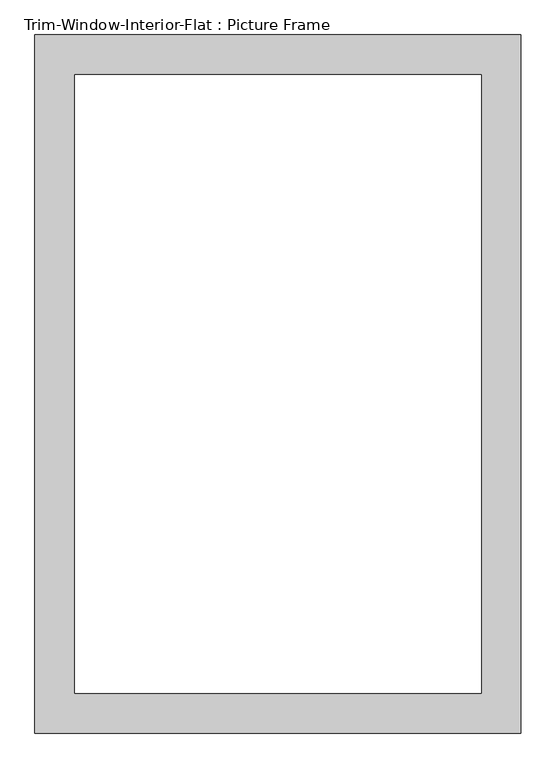
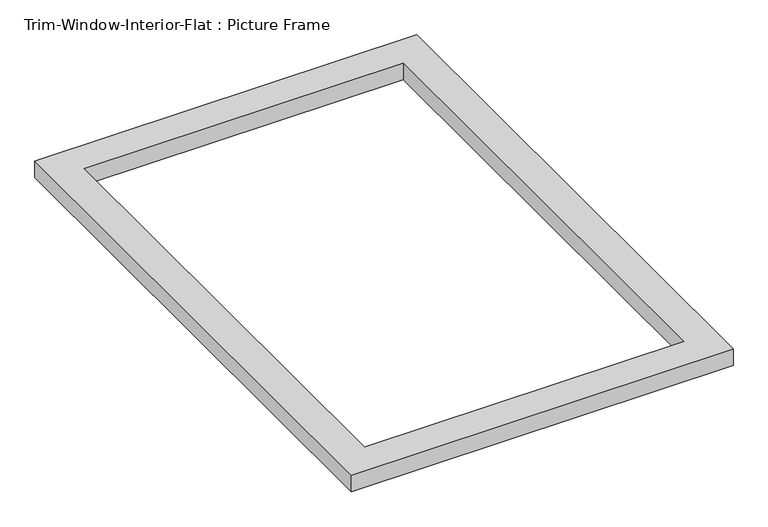
"""IFC4 building model written with IfcOpenShell, lengths in millimetres: proxy geometry, Trim-Window-Interior-Flat : Picture Frame."""

from ifc_helpers import new_model, si_unit, origin, origin_with_axes, place, context, project, spatial, polyline, outline, extrude, source, transform, mapped, element, save


def trim_window_interior_flat_picture_frame_d485c387(model_context):
    return source(origin(), model_context, "Body", "SweptSolid", [
        extrude(outline(polyline([(349.25, 44.45), (349.25, -958.85), (-349.25, -958.85), (-349.25, 44.45), (349.25, 44.45)]), holes=[polyline([(292.1, -12.7), (-292.1, -12.7), (-292.1, -901.7), (292.1, -901.7), (292.1, -12.7)])]), origin_with_axes(), (0.0, 0.0, 1.0), 31.75),
    ])


if __name__ == "__main__":
    model = new_model("IFC4")
    model_context = context("Model", 3, world=origin())
    ifc_project = project(units=[si_unit("LENGTHUNIT", "METRE", prefix="MILLI")], contexts=[model_context])
    site = spatial("IfcSite", under=ifc_project)
    building = spatial("IfcBuilding", under=site)
    placement = place(None, origin())
    trim_window_interior_flat_picture_frame_shape = trim_window_interior_flat_picture_frame_d485c387(model_context)
    element("IfcBuildingElementProxy", 1, Name="Trim-Window-Interior-Flat : Picture Frame", ObjectType="Trim-Window-Interior-Flat : Picture Frame", at=placement, inside=building, context=model_context, shape_type="MappedRepresentation", body=[
        mapped(trim_window_interior_flat_picture_frame_shape, transform((0.0, 0.0, 0.0), x_axis=(1.0, 0.0, 0.0), y_axis=(0.0, 1.0, 0.0), z_axis=(0.0, 0.0, 1.0))),
    ])
    save(model, "model.ifc")

# Revit data of these elements
# Type "Trim-Window-Interior-Flat : Picture Frame"
#   Trim Thickness_Picture Frame = 0' - 1 1/4"
#   Trim Width = 0' - 2 1/4"
#   Trim Thickness_with Sill = 0' - 0 3/4"
#   Sill Thickness = 0' - 1 1/4"
#   Opening Width [instance default] = 2' - 0"
#   Opening Height [instance default] = 3' - 0"
#   Default Elevation = 4' - 0"
#   Sill = no
#   Picture Frame = yes
#   Trim Material [instance default] = none
# Element 1 (IfcBuildingElementProxy, "Trim-Window-Interior-Flat : Picture Frame")
#   Trim Material = Wood - Stained
#   Materials on its faces: "Wood - Stained"
# Materials
#   "Wood - Stained": class "Wood", colour RGB 224 178 126, transparency 0, Cost = 0
